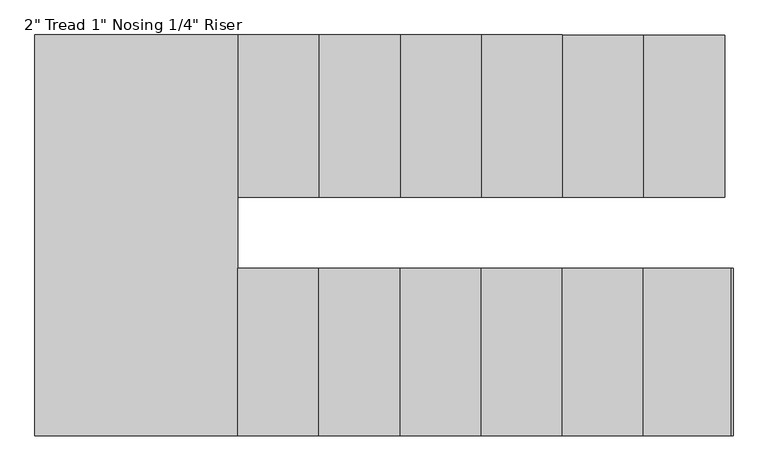
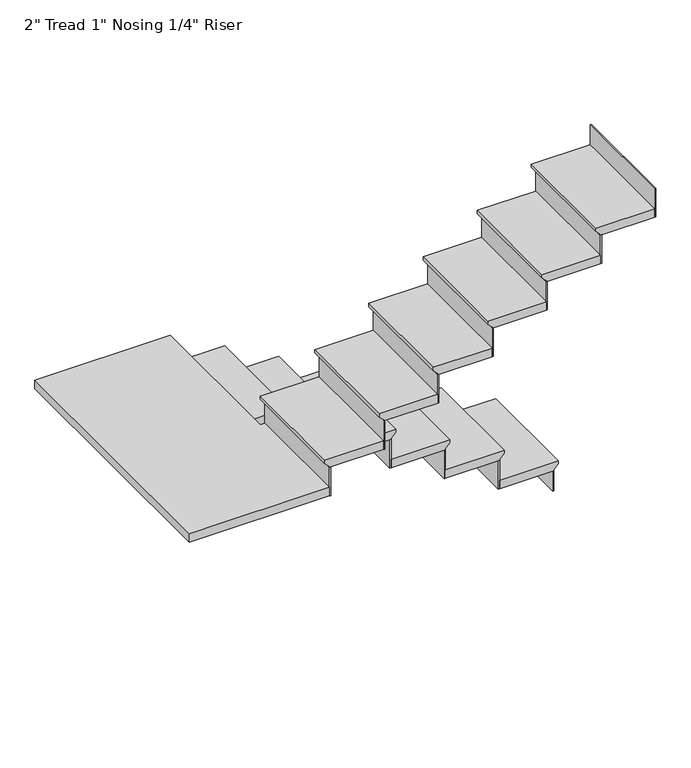
"""IFC4 building model written with IfcOpenShell, lengths in millimetres: stair flight geometry."""

from ifc_helpers import new_model, si_unit, origin, place, context, project, spatial, faceted_brep, source, transform, mapped, element, save


def stair_flight_6e983af9(model_context):
    return source(origin(), model_context, "Body", "Brep", [
        faceted_brep([(-2968.8120155, -2170.0065691, 16152.2833333), (-2968.8120155, -2170.0065691, 16171.3333333), (-2968.8120155, -2779.6065691, 16171.3333333), (-2968.8120155, -2779.6065691, 16152.2833333), (-2994.2120155, -2170.0065691, 16126.8833333), (-2994.2120155, -2779.6065691, 16126.8833333), (-3299.0120155, -2170.0065691, 16171.3333333), (-3299.0120155, -2779.6065691, 16171.3333333), (-2994.2120155, -2779.6065691, 16120.5333333), (-3299.0120155, -2779.6065691, 16120.5333333), (-3299.0120155, -2170.0065691, 16120.5333333), (-2994.2120155, -2170.0065691, 16120.5333333)], [[[0, 1, 2, 3]], [[4, 0, 3, 5]], [[2, 1, 6, 7]], [[8, 9, 10, 11]], [[2, 7, 9, 8, 5, 3]], [[8, 11, 4, 5]], [[6, 1, 0, 4, 11, 10]], [[7, 6, 10, 9]]]),
        faceted_brep([(-2994.2120155, -2170.0065691, 16120.5333333), (-2994.2120155, -2170.0065691, 16002.0), (-3000.5620155, -2170.0065691, 16002.0), (-3000.5620155, -2170.0065691, 16120.5333333), (-2994.2120155, -2779.6065691, 16120.5333333), (-3000.5620155, -2779.6065691, 16120.5333333), (-3000.5620155, -2779.6065691, 16002.0), (-2994.2120155, -2779.6065691, 16002.0)], [[[0, 1, 2, 3]], [[4, 5, 6, 7]], [[1, 0, 4, 7]], [[2, 1, 7, 6]], [[3, 2, 6, 5]], [[0, 3, 5, 4]]]),
        faceted_brep([(-3299.0120155, -2170.0065691, 16289.8666667), (-3299.0120155, -2170.0065691, 16120.5333333), (-3305.3620155, -2170.0065691, 16120.5333333), (-3305.3620155, -2170.0065691, 16289.8666667), (-3299.0120155, -2779.6065691, 16289.8666667), (-3305.3620155, -2779.6065691, 16289.8666667), (-3305.3620155, -2779.6065691, 16120.5333333), (-3299.0120155, -2779.6065691, 16120.5333333)], [[[0, 1, 2, 3]], [[4, 5, 6, 7]], [[1, 0, 4, 7]], [[2, 1, 7, 6]], [[3, 2, 6, 5]], [[0, 3, 5, 4]]]),
        faceted_brep([(-3273.6120155, -2779.6065691, 16340.6666667), (-3273.6120155, -2170.0065691, 16340.6666667), (-3603.8120155, -2170.0065691, 16340.6666667), (-3603.8120155, -2779.6065691, 16340.6666667), (-3299.0120155, -2779.6065691, 16289.8666667), (-3603.8120155, -2779.6065691, 16289.8666667), (-3603.8120155, -2170.0065691, 16289.8666667), (-3299.0120155, -2170.0065691, 16289.8666667), (-3299.0120155, -2779.6065691, 16296.2166667), (-3273.6120155, -2779.6065691, 16321.6166667), (-3299.0120155, -2170.0065691, 16296.2166667), (-3273.6120155, -2170.0065691, 16321.6166667)], [[[0, 1, 2, 3]], [[4, 5, 6, 7]], [[0, 3, 5, 4, 8, 9]], [[4, 7, 10, 8]], [[2, 1, 11, 10, 7, 6]], [[3, 2, 6, 5]], [[11, 1, 0, 9]], [[10, 11, 9, 8]]]),
        faceted_brep([(-3603.8120155, -2170.0065691, 16459.2), (-3603.8120155, -2170.0065691, 16289.8666667), (-3610.1620155, -2170.0065691, 16289.8666667), (-3610.1620155, -2170.0065691, 16459.2), (-3603.8120155, -2779.6065691, 16459.2), (-3610.1620155, -2779.6065691, 16459.2), (-3610.1620155, -2779.6065691, 16289.8666667), (-3603.8120155, -2779.6065691, 16289.8666667)], [[[0, 1, 2, 3]], [[4, 5, 6, 7]], [[1, 0, 4, 7]], [[2, 1, 7, 6]], [[3, 2, 6, 5]], [[0, 3, 5, 4]]]),
        faceted_brep([(-3578.4120155, -2779.6065691, 16510.0), (-3578.4120155, -2170.0065691, 16510.0), (-3908.6120155, -2170.0065691, 16510.0), (-3908.6120155, -2779.6065691, 16510.0), (-3603.8120155, -2779.6065691, 16459.2), (-3908.6120155, -2779.6065691, 16459.2), (-3908.6120155, -2170.0065691, 16459.2), (-3603.8120155, -2170.0065691, 16459.2), (-3603.8120155, -2779.6065691, 16465.55), (-3578.4120155, -2779.6065691, 16490.95), (-3603.8120155, -2170.0065691, 16465.55), (-3578.4120155, -2170.0065691, 16490.95)], [[[0, 1, 2, 3]], [[4, 5, 6, 7]], [[0, 3, 5, 4, 8, 9]], [[4, 7, 10, 8]], [[2, 1, 11, 10, 7, 6]], [[3, 2, 6, 5]], [[11, 1, 0, 9]], [[10, 11, 9, 8]]]),
        faceted_brep([(-3908.6120155, -2170.0065691, 16628.5333333), (-3908.6120155, -2170.0065691, 16459.2), (-3914.9620155, -2170.0065691, 16459.2), (-3914.9620155, -2170.0065691, 16628.5333333), (-3908.6120155, -2779.6065691, 16628.5333333), (-3914.9620155, -2779.6065691, 16628.5333333), (-3914.9620155, -2779.6065691, 16459.2), (-3908.6120155, -2779.6065691, 16459.2)], [[[0, 1, 2, 3]], [[4, 5, 6, 7]], [[1, 0, 4, 7]], [[2, 1, 7, 6]], [[3, 2, 6, 5]], [[0, 3, 5, 4]]]),
        faceted_brep([(-3883.2120155, -2779.6065691, 16679.3333333), (-3883.2120155, -2170.0065691, 16679.3333333), (-4213.4120155, -2170.0065691, 16679.3333333), (-4213.4120155, -2779.6065691, 16679.3333333), (-3908.6120155, -2779.6065691, 16628.5333333), (-4213.4120155, -2779.6065691, 16628.5333333), (-4213.4120155, -2170.0065691, 16628.5333333), (-3908.6120155, -2170.0065691, 16628.5333333), (-3908.6120155, -2779.6065691, 16634.8833333), (-3883.2120155, -2779.6065691, 16660.2833333), (-3908.6120155, -2170.0065691, 16634.8833333), (-3883.2120155, -2170.0065691, 16660.2833333)], [[[0, 1, 2, 3]], [[4, 5, 6, 7]], [[0, 3, 5, 4, 8, 9]], [[4, 7, 10, 8]], [[2, 1, 11, 10, 7, 6]], [[3, 2, 6, 5]], [[11, 1, 0, 9]], [[10, 11, 9, 8]]]),
        faceted_brep([(-4213.4120155, -2170.0065691, 16797.8666667), (-4213.4120155, -2170.0065691, 16628.5333333), (-4219.7620155, -2170.0065691, 16628.5333333), (-4219.7620155, -2170.0065691, 16797.8666667), (-4213.4120155, -2779.6065691, 16797.8666667), (-4219.7620155, -2779.6065691, 16797.8666667), (-4219.7620155, -2779.6065691, 16628.5333333), (-4213.4120155, -2779.6065691, 16628.5333333)], [[[0, 1, 2, 3]], [[4, 5, 6, 7]], [[1, 0, 4, 7]], [[2, 1, 7, 6]], [[3, 2, 6, 5]], [[0, 3, 5, 4]]]),
        faceted_brep([(-4188.0120155, -2779.6065691, 16848.6666667), (-4188.0120155, -2170.0065691, 16848.6666667), (-4518.2120155, -2170.0065691, 16848.6666667), (-4518.2120155, -2779.6065691, 16848.6666667), (-4213.4120155, -2779.6065691, 16797.8666667), (-4518.2120155, -2779.6065691, 16797.8666667), (-4518.2120155, -2170.0065691, 16797.8666667), (-4213.4120155, -2170.0065691, 16797.8666667), (-4213.4120155, -2779.6065691, 16804.2166667), (-4188.0120155, -2779.6065691, 16829.6166667), (-4213.4120155, -2170.0065691, 16804.2166667), (-4188.0120155, -2170.0065691, 16829.6166667)], [[[0, 1, 2, 3]], [[4, 5, 6, 7]], [[0, 3, 5, 4, 8, 9]], [[4, 7, 10, 8]], [[2, 1, 11, 10, 7, 6]], [[3, 2, 6, 5]], [[11, 1, 0, 9]], [[10, 11, 9, 8]]]),
        faceted_brep([(-4518.2120155, -2170.0065691, 16967.2), (-4518.2120155, -2170.0065691, 16797.8666667), (-4524.5620155, -2170.0065691, 16797.8666667), (-4524.5620155, -2170.0065691, 16967.2), (-4518.2120155, -2779.6065691, 16967.2), (-4524.5620155, -2779.6065691, 16967.2), (-4524.5620155, -2779.6065691, 16797.8666667), (-4518.2120155, -2779.6065691, 16797.8666667)], [[[0, 1, 2, 3]], [[4, 5, 6, 7]], [[1, 0, 4, 7]], [[2, 1, 7, 6]], [[3, 2, 6, 5]], [[0, 3, 5, 4]]]),
        faceted_brep([(-4492.8120155, -2779.6065691, 17018.0), (-4492.8120155, -2170.0065691, 17018.0), (-4823.0120155, -2170.0065691, 17018.0), (-4823.0120155, -2779.6065691, 17018.0), (-4518.2120155, -2779.6065691, 16967.2), (-4823.0120155, -2779.6065691, 16967.2), (-4823.0120155, -2170.0065691, 16967.2), (-4518.2120155, -2170.0065691, 16967.2), (-4518.2120155, -2779.6065691, 16973.55), (-4492.8120155, -2779.6065691, 16998.95), (-4518.2120155, -2170.0065691, 16973.55), (-4492.8120155, -2170.0065691, 16998.95)], [[[0, 1, 2, 3]], [[4, 5, 6, 7]], [[0, 3, 5, 4, 8, 9]], [[4, 7, 10, 8]], [[2, 1, 11, 10, 7, 6]], [[3, 2, 6, 5]], [[11, 1, 0, 9]], [[10, 11, 9, 8]]]),
        faceted_brep([(-4823.0120155, -2170.0065691, 17136.5333333), (-4823.0120155, -2170.0065691, 16967.2), (-4829.3620155, -2170.0065691, 16967.2), (-4829.3620155, -2170.0065691, 17136.5333333), (-4823.0120155, -2779.6065691, 17136.5333333), (-4829.3620155, -2779.6065691, 17136.5333333), (-4829.3620155, -2779.6065691, 16967.2), (-4823.0120155, -2779.6065691, 16967.2)], [[[0, 1, 2, 3]], [[4, 5, 6, 7]], [[1, 0, 4, 7]], [[2, 1, 7, 6]], [[3, 2, 6, 5]], [[0, 3, 5, 4]]]),
        faceted_brep([(-4772.2120155, -3046.3065691, 17187.3333333), (-4797.6120155, -3046.3065691, 17187.3333333), (-4797.6120155, -2170.0065691, 17187.3333333), (-5559.6120155, -2170.0065691, 17187.3333333), (-5559.6120155, -3674.9565691, 17187.3333333), (-4772.2120155, -3674.9565691, 17187.3333333), (-4797.6120155, -3046.3065691, 17136.5333333), (-4772.2120155, -3046.3065691, 17136.5333333), (-4772.2120155, -3674.9565691, 17136.5333333), (-5559.6120155, -3674.9565691, 17136.5333333), (-5559.6120155, -2170.0065691, 17136.5333333), (-4823.0120155, -2170.0065691, 17136.5333333), (-4823.0120155, -2779.6065691, 17136.5333333), (-4797.6120155, -2779.6065691, 17136.5333333), (-4797.6120155, -2779.6065691, 17168.2833333), (-4797.6120155, -2170.0065691, 17168.2833333), (-4823.0120155, -2779.6065691, 17142.8833333), (-4823.0120155, -2170.0065691, 17142.8833333)], [[[0, 1, 2, 3, 4, 5]], [[6, 7, 8, 9, 10, 11, 12, 13]], [[1, 0, 7, 6]], [[2, 1, 6, 13, 14, 15]], [[13, 12, 16, 14]], [[12, 11, 17, 16]], [[3, 2, 15, 17, 11, 10]], [[4, 3, 10, 9]], [[5, 4, 9, 8]], [[0, 5, 8, 7]], [[17, 15, 14, 16]]]),
        faceted_brep([(-4772.2120155, -3674.9565691, 17305.8666667), (-4772.2120155, -3674.9565691, 17136.5333333), (-4765.8620155, -3674.9565691, 17136.5333333), (-4765.8620155, -3674.9565691, 17305.8666667), (-4772.2120155, -3046.3065691, 17305.8666667), (-4765.8620155, -3046.3065691, 17305.8666667), (-4765.8620155, -3046.3065691, 17136.5333333), (-4772.2120155, -3046.3065691, 17136.5333333)], [[[0, 1, 2, 3]], [[4, 5, 6, 7]], [[1, 0, 4, 7]], [[2, 1, 7, 6]], [[3, 2, 6, 5]], [[0, 3, 5, 4]]]),
        faceted_brep([(-4797.6120155, -3046.3065691, 17356.6666667), (-4797.6120155, -3674.9565691, 17356.6666667), (-4467.4120155, -3674.9565691, 17356.6666667), (-4467.4120155, -3046.3065691, 17356.6666667), (-4772.2120155, -3046.3065691, 17305.8666667), (-4467.4120155, -3046.3065691, 17305.8666667), (-4467.4120155, -3674.9565691, 17305.8666667), (-4772.2120155, -3674.9565691, 17305.8666667), (-4772.2120155, -3046.3065691, 17312.2166667), (-4797.6120155, -3046.3065691, 17337.6166667), (-4772.2120155, -3674.9565691, 17312.2166667), (-4797.6120155, -3674.9565691, 17337.6166667)], [[[0, 1, 2, 3]], [[4, 5, 6, 7]], [[0, 3, 5, 4, 8, 9]], [[4, 7, 10, 8]], [[2, 1, 11, 10, 7, 6]], [[3, 2, 6, 5]], [[11, 1, 0, 9]], [[10, 11, 9, 8]]]),
        faceted_brep([(-4467.4120155, -3674.9565691, 17475.2), (-4467.4120155, -3674.9565691, 17305.8666667), (-4461.0620155, -3674.9565691, 17305.8666667), (-4461.0620155, -3674.9565691, 17475.2), (-4467.4120155, -3046.3065691, 17475.2), (-4461.0620155, -3046.3065691, 17475.2), (-4461.0620155, -3046.3065691, 17305.8666667), (-4467.4120155, -3046.3065691, 17305.8666667)], [[[0, 1, 2, 3]], [[4, 5, 6, 7]], [[1, 0, 4, 7]], [[2, 1, 7, 6]], [[3, 2, 6, 5]], [[0, 3, 5, 4]]]),
        faceted_brep([(-4492.8120155, -3046.3065691, 17526.0), (-4492.8120155, -3674.9565691, 17526.0), (-4162.6120155, -3674.9565691, 17526.0), (-4162.6120155, -3046.3065691, 17526.0), (-4467.4120155, -3046.3065691, 17475.2), (-4162.6120155, -3046.3065691, 17475.2), (-4162.6120155, -3674.9565691, 17475.2), (-4467.4120155, -3674.9565691, 17475.2), (-4467.4120155, -3046.3065691, 17481.55), (-4492.8120155, -3046.3065691, 17506.95), (-4467.4120155, -3674.9565691, 17481.55), (-4492.8120155, -3674.9565691, 17506.95)], [[[0, 1, 2, 3]], [[4, 5, 6, 7]], [[0, 3, 5, 4, 8, 9]], [[4, 7, 10, 8]], [[2, 1, 11, 10, 7, 6]], [[3, 2, 6, 5]], [[11, 1, 0, 9]], [[10, 11, 9, 8]]]),
        faceted_brep([(-4162.6120155, -3674.9565691, 17644.5333333), (-4162.6120155, -3674.9565691, 17475.2), (-4156.2620155, -3674.9565691, 17475.2), (-4156.2620155, -3674.9565691, 17644.5333333), (-4162.6120155, -3046.3065691, 17644.5333333), (-4156.2620155, -3046.3065691, 17644.5333333), (-4156.2620155, -3046.3065691, 17475.2), (-4162.6120155, -3046.3065691, 17475.2)], [[[0, 1, 2, 3]], [[4, 5, 6, 7]], [[1, 0, 4, 7]], [[2, 1, 7, 6]], [[3, 2, 6, 5]], [[0, 3, 5, 4]]]),
        faceted_brep([(-4188.0120155, -3046.3065691, 17695.3333333), (-4188.0120155, -3674.9565691, 17695.3333333), (-3857.8120155, -3674.9565691, 17695.3333333), (-3857.8120155, -3046.3065691, 17695.3333333), (-4162.6120155, -3046.3065691, 17644.5333333), (-3857.8120155, -3046.3065691, 17644.5333333), (-3857.8120155, -3674.9565691, 17644.5333333), (-4162.6120155, -3674.9565691, 17644.5333333), (-4162.6120155, -3046.3065691, 17650.8833333), (-4188.0120155, -3046.3065691, 17676.2833333), (-4162.6120155, -3674.9565691, 17650.8833333), (-4188.0120155, -3674.9565691, 17676.2833333)], [[[0, 1, 2, 3]], [[4, 5, 6, 7]], [[0, 3, 5, 4, 8, 9]], [[4, 7, 10, 8]], [[2, 1, 11, 10, 7, 6]], [[3, 2, 6, 5]], [[11, 1, 0, 9]], [[10, 11, 9, 8]]]),
        faceted_brep([(-3857.8120155, -3674.9565691, 17813.8666667), (-3857.8120155, -3674.9565691, 17644.5333333), (-3851.4620155, -3674.9565691, 17644.5333333), (-3851.4620155, -3674.9565691, 17813.8666667), (-3857.8120155, -3046.3065691, 17813.8666667), (-3851.4620155, -3046.3065691, 17813.8666667), (-3851.4620155, -3046.3065691, 17644.5333333), (-3857.8120155, -3046.3065691, 17644.5333333)], [[[0, 1, 2, 3]], [[4, 5, 6, 7]], [[1, 0, 4, 7]], [[2, 1, 7, 6]], [[3, 2, 6, 5]], [[0, 3, 5, 4]]]),
        faceted_brep([(-3883.2120155, -3046.3065691, 17864.6666667), (-3883.2120155, -3674.9565691, 17864.6666667), (-3553.0120155, -3674.9565691, 17864.6666667), (-3553.0120155, -3046.3065691, 17864.6666667), (-3857.8120155, -3046.3065691, 17813.8666667), (-3553.0120155, -3046.3065691, 17813.8666667), (-3553.0120155, -3674.9565691, 17813.8666667), (-3857.8120155, -3674.9565691, 17813.8666667), (-3857.8120155, -3046.3065691, 17820.2166667), (-3883.2120155, -3046.3065691, 17845.6166667), (-3857.8120155, -3674.9565691, 17820.2166667), (-3883.2120155, -3674.9565691, 17845.6166667)], [[[0, 1, 2, 3]], [[4, 5, 6, 7]], [[0, 3, 5, 4, 8, 9]], [[4, 7, 10, 8]], [[2, 1, 11, 10, 7, 6]], [[3, 2, 6, 5]], [[11, 1, 0, 9]], [[10, 11, 9, 8]]]),
        faceted_brep([(-3553.0120155, -3674.9565691, 17983.2), (-3553.0120155, -3674.9565691, 17813.8666667), (-3546.6620155, -3674.9565691, 17813.8666667), (-3546.6620155, -3674.9565691, 17983.2), (-3553.0120155, -3046.3065691, 17983.2), (-3546.6620155, -3046.3065691, 17983.2), (-3546.6620155, -3046.3065691, 17813.8666667), (-3553.0120155, -3046.3065691, 17813.8666667)], [[[0, 1, 2, 3]], [[4, 5, 6, 7]], [[1, 0, 4, 7]], [[2, 1, 7, 6]], [[3, 2, 6, 5]], [[0, 3, 5, 4]]]),
        faceted_brep([(-3578.4120155, -3046.3065691, 18034.0), (-3578.4120155, -3674.9565691, 18034.0), (-3248.2120155, -3674.9565691, 18034.0), (-3248.2120155, -3046.3065691, 18034.0), (-3553.0120155, -3046.3065691, 17983.2), (-3248.2120155, -3046.3065691, 17983.2), (-3248.2120155, -3674.9565691, 17983.2), (-3553.0120155, -3674.9565691, 17983.2), (-3553.0120155, -3046.3065691, 17989.55), (-3578.4120155, -3046.3065691, 18014.95), (-3553.0120155, -3674.9565691, 17989.55), (-3578.4120155, -3674.9565691, 18014.95)], [[[0, 1, 2, 3]], [[4, 5, 6, 7]], [[0, 3, 5, 4, 8, 9]], [[4, 7, 10, 8]], [[2, 1, 11, 10, 7, 6]], [[3, 2, 6, 5]], [[11, 1, 0, 9]], [[10, 11, 9, 8]]]),
        faceted_brep([(-3248.2120155, -3674.9565691, 18152.5333333), (-3248.2120155, -3674.9565691, 17983.2), (-3241.8620155, -3674.9565691, 17983.2), (-3241.8620155, -3674.9565691, 18152.5333333), (-3248.2120155, -3046.3065691, 18152.5333333), (-3241.8620155, -3046.3065691, 18152.5333333), (-3241.8620155, -3046.3065691, 17983.2), (-3248.2120155, -3046.3065691, 17983.2)], [[[0, 1, 2, 3]], [[4, 5, 6, 7]], [[1, 0, 4, 7]], [[2, 1, 7, 6]], [[3, 2, 6, 5]], [[0, 3, 5, 4]]]),
        faceted_brep([(-2943.4120155, -3674.9565691, 18321.8666667), (-2943.4120155, -3674.9565691, 18152.5333333), (-2937.0620155, -3674.9565691, 18152.5333333), (-2937.0620155, -3674.9565691, 18321.8666667), (-2943.4120155, -3046.3065691, 18321.8666667), (-2937.0620155, -3046.3065691, 18321.8666667), (-2937.0620155, -3046.3065691, 18152.5333333), (-2943.4120155, -3046.3065691, 18152.5333333)], [[[0, 1, 2, 3]], [[4, 5, 6, 7]], [[1, 0, 4, 7]], [[2, 1, 7, 6]], [[3, 2, 6, 5]], [[0, 3, 5, 4]]]),
        faceted_brep([(-3273.6120155, -3046.3065691, 18203.3333333), (-3273.6120155, -3674.9565691, 18203.3333333), (-2943.4120155, -3674.9565691, 18203.3333333), (-2943.4120155, -3046.3065691, 18203.3333333), (-3248.2120155, -3046.3065691, 18152.5333333), (-2943.4120155, -3046.3065691, 18152.5333333), (-2943.4120155, -3674.9565691, 18152.5333333), (-3248.2120155, -3674.9565691, 18152.5333333), (-3248.2120155, -3046.3065691, 18158.8833333), (-3273.6120155, -3046.3065691, 18184.2833333), (-3248.2120155, -3674.9565691, 18158.8833333), (-3273.6120155, -3674.9565691, 18184.2833333)], [[[0, 1, 2, 3]], [[4, 5, 6, 7]], [[0, 3, 5, 4, 8, 9]], [[4, 7, 10, 8]], [[2, 1, 11, 10, 7, 6]], [[3, 2, 6, 5]], [[11, 1, 0, 9]], [[10, 11, 9, 8]]]),
    ])


if __name__ == "__main__":
    model = new_model("IFC4")
    model_context = context("Model", 3, world=origin())
    ifc_project = project(units=[si_unit("LENGTHUNIT", "METRE", prefix="MILLI")], contexts=[model_context])
    site = spatial("IfcSite", under=ifc_project)
    building = spatial("IfcBuilding", under=site)
    placement = place(None, origin())
    stair_flight_shape = stair_flight_6e983af9(model_context)
    element("IfcStairFlight", 1, ObjectType="2\" Tread 1\" Nosing 1/4\" Riser", at=placement, inside=building, context=model_context, shape_type="MappedRepresentation", body=[
        mapped(stair_flight_shape, transform((0.0, 0.0, 0.0), x_axis=(1.0, 0.0, 0.0), y_axis=(0.0, 1.0, 0.0), z_axis=(0.0, 0.0, 1.0))),
    ])
    save(model, "model.ifc")
